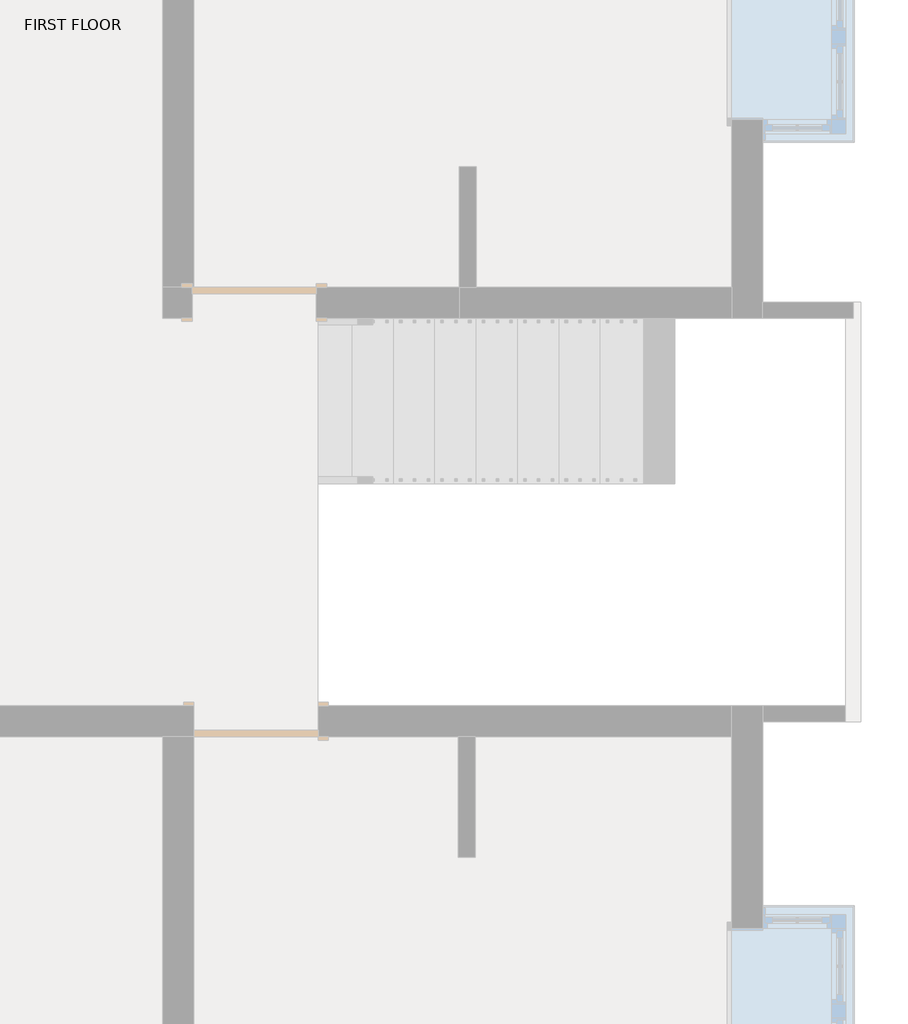
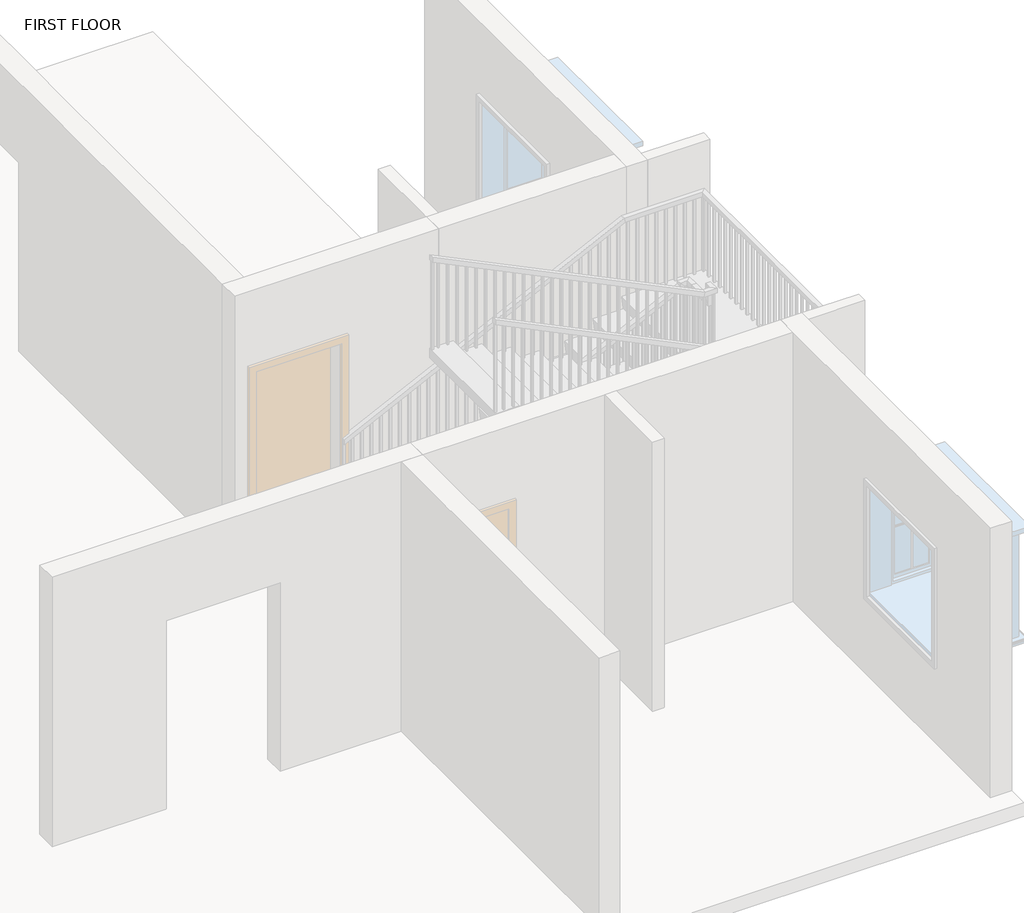
# One storey, part 5 of 6: 1 railing.
"""IFC4 building model written with IfcOpenShell, lengths in millimetres."""

from ifc_helpers import new_model, si_unit, frame, origin, place, context, project, spatial, polyline, outline, extrude, faceted_brep, element, save

model = new_model("IFC4")

# Units and contexts
model_context = context("Model", 3, world=origin())
ifc_project = project(units=[si_unit("LENGTHUNIT", "METRE", prefix="MILLI")], contexts=[model_context])

# Site, building, storey
site = spatial("IfcSite", under=ifc_project)
building = spatial("IfcBuilding", under=site)
storey = spatial("IfcBuildingStorey", under=building, Name="FIRST FLOOR", Elevation=3200.4)

# Railing
placement = place(None, origin())
element("IfcRailing", 1, ObjectType="Handrail - Rectangular", at=placement, inside=storey, context=model_context, shape_type="SolidModel", body=[
    faceted_brep([(3126.2584916, 220.733346, 4260.2727273), (3126.2584916, 220.733346, 4203.7956113), (3126.2584916, 169.933346, 4203.7956113), (3126.2584916, 169.933346, 4260.2727273), (6120.7829507, 220.733346, 5715.0), (6132.4691705, 220.733346, 5664.2), (6132.4691705, 169.933346, 5664.2), (6120.7829507, 169.933346, 5715.0), (7009.1350459, 220.733346, 5715.0), (7009.1350459, 220.733346, 5664.2), (6958.3350459, 169.933346, 5664.2), (6958.3350459, 169.933346, 5715.0), (7009.1350459, -2636.766654, 5715.0), (7009.1350459, -2636.766654, 5664.2), (6958.3350459, -2585.966654, 5664.2), (6958.3350459, -2585.966654, 5715.0), (6420.2353966, -2636.766654, 5715.0), (6408.5491768, -2636.766654, 5664.2), (6408.5491768, -2585.966654, 5664.2), (6420.2353966, -2585.966654, 5715.0), (3126.2584916, -2636.766654, 7315.2), (3126.2584916, -2585.966654, 7315.2), (3126.2584916, -2585.966654, 7258.722884), (3126.2584916, -2636.766654, 7258.722884)], [[[0, 1, 2, 3]], [[1, 0, 4, 5]], [[2, 1, 5, 6]], [[3, 2, 6, 7]], [[0, 3, 7, 4]], [[5, 4, 8, 9]], [[6, 5, 9, 10]], [[7, 6, 10, 11]], [[4, 7, 11, 8]], [[9, 8, 12, 13]], [[10, 9, 13, 14]], [[11, 10, 14, 15]], [[8, 11, 15, 12]], [[13, 12, 16, 17]], [[14, 13, 17, 18]], [[15, 14, 18, 19]], [[12, 15, 19, 16]], [[20, 21, 22, 23]], [[17, 16, 20, 23]], [[18, 17, 23, 22]], [[19, 18, 22, 21]], [[16, 19, 21, 20]]]),
    extrude(outline(polyline([(7215.6077556, 3215.0100459), (6255.3272727, 3215.0100459), (6255.3272727, 3234.0600459), (7206.3533465, 3234.0600459), (7215.6077556, 3215.0100459)])), frame((0.0, -2620.891654, 0.0), z_axis=(0.0, 1.0, 0.0), x_axis=(0.0, 0.0, 1.0)), (0.0, 0.0, 1.0), 19.05),
    extrude(outline(polyline([(7166.2509068, 3316.6100459), (6255.3272727, 3316.6100459), (6255.3272727, 3335.6600459), (7156.9964977, 3335.6600459), (7166.2509068, 3316.6100459)])), frame((0.0, -2620.891654, 0.0), z_axis=(0.0, 1.0, 0.0), x_axis=(0.0, 0.0, 1.0)), (0.0, 0.0, 1.0), 19.05),
    extrude(outline(polyline([(7116.894058, 3418.2100459), (6109.8545455, 3418.2100459), (6109.8545455, 3437.2600459), (7107.6396489, 3437.2600459), (7116.894058, 3418.2100459)])), frame((0.0, -2620.891654, 0.0), z_axis=(0.0, 1.0, 0.0), x_axis=(0.0, 0.0, 1.0)), (0.0, 0.0, 1.0), 19.05),
    extrude(outline(polyline([(7067.5372093, 3519.8100459), (6109.8545455, 3519.8100459), (6109.8545455, 3538.8600459), (7058.2828001, 3538.8600459), (7067.5372093, 3519.8100459)])), frame((0.0, -2620.891654, 0.0), z_axis=(0.0, 1.0, 0.0), x_axis=(0.0, 0.0, 1.0)), (0.0, 0.0, 1.0), 19.05),
    extrude(outline(polyline([(7018.1803605, 3621.4100459), (6109.8545455, 3621.4100459), (6109.8545455, 3640.4600459), (7008.9259513, 3640.4600459), (7018.1803605, 3621.4100459)])), frame((0.0, -2620.891654, 0.0), z_axis=(0.0, 1.0, 0.0), x_axis=(0.0, 0.0, 1.0)), (0.0, 0.0, 1.0), 19.05),
    extrude(outline(polyline([(6968.8235117, 3723.0100459), (5964.3818182, 3723.0100459), (5964.3818182, 3742.0600459), (6959.5691025, 3742.0600459), (6968.8235117, 3723.0100459)])), frame((0.0, -2620.891654, 0.0), z_axis=(0.0, 1.0, 0.0), x_axis=(0.0, 0.0, 1.0)), (0.0, 0.0, 1.0), 19.05),
    extrude(outline(polyline([(6919.4666629, 3824.6100459), (5964.3818182, 3824.6100459), (5964.3818182, 3843.6600459), (6910.2122538, 3843.6600459), (6919.4666629, 3824.6100459)])), frame((0.0, -2620.891654, 0.0), z_axis=(0.0, 1.0, 0.0), x_axis=(0.0, 0.0, 1.0)), (0.0, 0.0, 1.0), 19.05),
    extrude(outline(polyline([(6870.1098141, 3926.2100459), (5964.3818182, 3926.2100459), (5964.3818182, 3945.2600459), (6860.855405, 3945.2600459), (6870.1098141, 3926.2100459)])), frame((0.0, -2620.891654, 0.0), z_axis=(0.0, 1.0, 0.0), x_axis=(0.0, 0.0, 1.0)), (0.0, 0.0, 1.0), 19.05),
    extrude(outline(polyline([(6820.7529653, 4027.8100459), (5818.9090909, 4027.8100459), (5818.9090909, 4046.8600459), (6811.4985562, 4046.8600459), (6820.7529653, 4027.8100459)])), frame((0.0, -2620.891654, 0.0), z_axis=(0.0, 1.0, 0.0), x_axis=(0.0, 0.0, 1.0)), (0.0, 0.0, 1.0), 19.05),
    extrude(outline(polyline([(6771.3961165, 4129.4100459), (5818.9090909, 4129.4100459), (5818.9090909, 4148.4600459), (6762.1417074, 4148.4600459), (6771.3961165, 4129.4100459)])), frame((0.0, -2620.891654, 0.0), z_axis=(0.0, 1.0, 0.0), x_axis=(0.0, 0.0, 1.0)), (0.0, 0.0, 1.0), 19.05),
    extrude(outline(polyline([(6722.0392678, 4231.0100459), (5818.9090909, 4231.0100459), (5818.9090909, 4250.0600459), (6712.7848586, 4250.0600459), (6722.0392678, 4231.0100459)])), frame((0.0, -2620.891654, 0.0), z_axis=(0.0, 1.0, 0.0), x_axis=(0.0, 0.0, 1.0)), (0.0, 0.0, 1.0), 19.05),
    extrude(outline(polyline([(6672.682419, 4332.6100459), (5673.4363636, 4332.6100459), (5673.4363636, 4351.6600459), (6663.4280098, 4351.6600459), (6672.682419, 4332.6100459)])), frame((0.0, -2620.891654, 0.0), z_axis=(0.0, 1.0, 0.0), x_axis=(0.0, 0.0, 1.0)), (0.0, 0.0, 1.0), 19.05),
    extrude(outline(polyline([(6623.3255702, 4434.2100459), (5673.4363636, 4434.2100459), (5673.4363636, 4453.2600459), (6614.071161, 4453.2600459), (6623.3255702, 4434.2100459)])), frame((0.0, -2620.891654, 0.0), z_axis=(0.0, 1.0, 0.0), x_axis=(0.0, 0.0, 1.0)), (0.0, 0.0, 1.0), 19.05),
    extrude(outline(polyline([(6573.9687214, 4535.8100459), (5673.4363636, 4535.8100459), (5673.4363636, 4554.8600459), (6564.7143123, 4554.8600459), (6573.9687214, 4535.8100459)])), frame((0.0, -2620.891654, 0.0), z_axis=(0.0, 1.0, 0.0), x_axis=(0.0, 0.0, 1.0)), (0.0, 0.0, 1.0), 19.05),
    extrude(outline(polyline([(6524.6118726, 4637.4100459), (5527.9636364, 4637.4100459), (5527.9636364, 4656.4600459), (6515.3574635, 4656.4600459), (6524.6118726, 4637.4100459)])), frame((0.0, -2620.891654, 0.0), z_axis=(0.0, 1.0, 0.0), x_axis=(0.0, 0.0, 1.0)), (0.0, 0.0, 1.0), 19.05),
    extrude(outline(polyline([(6475.2550238, 4739.0100459), (5527.9636364, 4739.0100459), (5527.9636364, 4758.0600459), (6466.0006147, 4758.0600459), (6475.2550238, 4739.0100459)])), frame((0.0, -2620.891654, 0.0), z_axis=(0.0, 1.0, 0.0), x_axis=(0.0, 0.0, 1.0)), (0.0, 0.0, 1.0), 19.05),
    extrude(outline(polyline([(6425.8981751, 4840.6100459), (5527.9636364, 4840.6100459), (5527.9636364, 4859.6600459), (6416.6437659, 4859.6600459), (6425.8981751, 4840.6100459)])), frame((0.0, -2620.891654, 0.0), z_axis=(0.0, 1.0, 0.0), x_axis=(0.0, 0.0, 1.0)), (0.0, 0.0, 1.0), 19.05),
    extrude(outline(polyline([(6376.5413263, 4942.2100459), (5382.4909091, 4942.2100459), (5382.4909091, 4961.2600459), (6367.2869171, 4961.2600459), (6376.5413263, 4942.2100459)])), frame((0.0, -2620.891654, 0.0), z_axis=(0.0, 1.0, 0.0), x_axis=(0.0, 0.0, 1.0)), (0.0, 0.0, 1.0), 19.05),
    extrude(outline(polyline([(6327.1844775, 5043.8100459), (5382.4909091, 5043.8100459), (5382.4909091, 5062.8600459), (6317.9300683, 5062.8600459), (6327.1844775, 5043.8100459)])), frame((0.0, -2620.891654, 0.0), z_axis=(0.0, 1.0, 0.0), x_axis=(0.0, 0.0, 1.0)), (0.0, 0.0, 1.0), 19.05),
    extrude(outline(polyline([(6277.8276287, 5145.4100459), (5382.4909091, 5145.4100459), (5382.4909091, 5164.4600459), (6268.5732196, 5164.4600459), (6277.8276287, 5145.4100459)])), frame((0.0, -2620.891654, 0.0), z_axis=(0.0, 1.0, 0.0), x_axis=(0.0, 0.0, 1.0)), (0.0, 0.0, 1.0), 19.05),
    extrude(outline(polyline([(6228.4707799, 5247.0100459), (5237.0181818, 5247.0100459), (5237.0181818, 5266.0600459), (6219.2163708, 5266.0600459), (6228.4707799, 5247.0100459)])), frame((0.0, -2620.891654, 0.0), z_axis=(0.0, 1.0, 0.0), x_axis=(0.0, 0.0, 1.0)), (0.0, 0.0, 1.0), 19.05),
    extrude(outline(polyline([(6179.1139311, 5348.6100459), (5237.0181818, 5348.6100459), (5237.0181818, 5367.6600459), (6169.859522, 5367.6600459), (6179.1139311, 5348.6100459)])), frame((0.0, -2620.891654, 0.0), z_axis=(0.0, 1.0, 0.0), x_axis=(0.0, 0.0, 1.0)), (0.0, 0.0, 1.0), 19.05),
    extrude(outline(polyline([(6129.7570823, 5450.2100459), (5237.0181818, 5450.2100459), (5237.0181818, 5469.2600459), (6120.5026732, 5469.2600459), (6129.7570823, 5450.2100459)])), frame((0.0, -2620.891654, 0.0), z_axis=(0.0, 1.0, 0.0), x_axis=(0.0, 0.0, 1.0)), (0.0, 0.0, 1.0), 19.05),
    extrude(outline(polyline([(6080.4002336, 5551.8100459), (5091.5454545, 5551.8100459), (5091.5454545, 5570.8600459), (6071.1458244, 5570.8600459), (6080.4002336, 5551.8100459)])), frame((0.0, -2620.891654, 0.0), z_axis=(0.0, 1.0, 0.0), x_axis=(0.0, 0.0, 1.0)), (0.0, 0.0, 1.0), 19.05),
    extrude(outline(polyline([(6031.0433848, 5653.4100459), (5091.5454545, 5653.4100459), (5091.5454545, 5672.4600459), (6021.7889756, 5672.4600459), (6031.0433848, 5653.4100459)])), frame((0.0, -2620.891654, 0.0), z_axis=(0.0, 1.0, 0.0), x_axis=(0.0, 0.0, 1.0)), (0.0, 0.0, 1.0), 19.05),
    extrude(outline(polyline([(5981.686536, 5755.0100459), (5091.5454545, 5755.0100459), (5091.5454545, 5774.0600459), (5972.4321268, 5774.0600459), (5981.686536, 5755.0100459)])), frame((0.0, -2620.891654, 0.0), z_axis=(0.0, 1.0, 0.0), x_axis=(0.0, 0.0, 1.0)), (0.0, 0.0, 1.0), 19.05),
    extrude(outline(polyline([(5932.3296872, 5856.6100459), (4946.0727273, 5856.6100459), (4946.0727273, 5875.6600459), (5923.0752781, 5875.6600459), (5932.3296872, 5856.6100459)])), frame((0.0, -2620.891654, 0.0), z_axis=(0.0, 1.0, 0.0), x_axis=(0.0, 0.0, 1.0)), (0.0, 0.0, 1.0), 19.05),
    extrude(outline(polyline([(5882.9728384, 5958.2100459), (4946.0727273, 5958.2100459), (4946.0727273, 5977.2600459), (5873.7184293, 5977.2600459), (5882.9728384, 5958.2100459)])), frame((0.0, -2620.891654, 0.0), z_axis=(0.0, 1.0, 0.0), x_axis=(0.0, 0.0, 1.0)), (0.0, 0.0, 1.0), 19.05),
    extrude(outline(polyline([(5833.6159896, 6059.8100459), (4946.0727273, 6059.8100459), (4946.0727273, 6078.8600459), (5824.3615805, 6078.8600459), (5833.6159896, 6059.8100459)])), frame((0.0, -2620.891654, 0.0), z_axis=(0.0, 1.0, 0.0), x_axis=(0.0, 0.0, 1.0)), (0.0, 0.0, 1.0), 19.05),
    extrude(outline(polyline([(5784.2591409, 6161.4100459), (4800.6, 6161.4100459), (4800.6, 6180.4600459), (5775.0047317, 6180.4600459), (5784.2591409, 6161.4100459)])), frame((0.0, -2620.891654, 0.0), z_axis=(0.0, 1.0, 0.0), x_axis=(0.0, 0.0, 1.0)), (0.0, 0.0, 1.0), 19.05),
    extrude(outline(polyline([(5734.9022921, 6263.0100459), (4800.6, 6263.0100459), (4800.6, 6282.0600459), (5725.6478829, 6282.0600459), (5734.9022921, 6263.0100459)])), frame((0.0, -2620.891654, 0.0), z_axis=(0.0, 1.0, 0.0), x_axis=(0.0, 0.0, 1.0)), (0.0, 0.0, 1.0), 19.05),
    extrude(outline(polyline([(5685.5454433, 6364.6100459), (4800.6, 6364.6100459), (4800.6, 6383.6600459), (5676.2910341, 6383.6600459), (5685.5454433, 6364.6100459)])), frame((0.0, -2620.891654, 0.0), z_axis=(0.0, 1.0, 0.0), x_axis=(0.0, 0.0, 1.0)), (0.0, 0.0, 1.0), 19.05),
    extrude(outline(polyline([(6485.2600459, -2620.891654), (6466.2100459, -2620.891654), (6466.2100459, -2601.841654), (6485.2600459, -2601.841654), (6485.2600459, -2620.891654)])), frame((0.0, 0.0, 4800.6), z_axis=(0.0, 0.0, 1.0), x_axis=(1.0, 0.0, 0.0)), (0.0, 0.0, 1.0), 863.6),
    extrude(outline(polyline([(6586.8600459, -2620.891654), (6567.8100459, -2620.891654), (6567.8100459, -2601.841654), (6586.8600459, -2601.841654), (6586.8600459, -2620.891654)])), frame((0.0, 0.0, 4800.6), z_axis=(0.0, 0.0, 1.0), x_axis=(1.0, 0.0, 0.0)), (0.0, 0.0, 1.0), 863.6),
    extrude(outline(polyline([(6688.4600459, -2620.891654), (6669.4100459, -2620.891654), (6669.4100459, -2601.841654), (6688.4600459, -2601.841654), (6688.4600459, -2620.891654)])), frame((0.0, 0.0, 4800.6), z_axis=(0.0, 0.0, 1.0), x_axis=(1.0, 0.0, 0.0)), (0.0, 0.0, 1.0), 863.6),
    extrude(outline(polyline([(6790.0600459, -2620.891654), (6771.0100459, -2620.891654), (6771.0100459, -2601.841654), (6790.0600459, -2601.841654), (6790.0600459, -2620.891654)])), frame((0.0, 0.0, 4800.6), z_axis=(0.0, 0.0, 1.0), x_axis=(1.0, 0.0, 0.0)), (0.0, 0.0, 1.0), 863.6),
    extrude(outline(polyline([(6891.6600459, -2620.891654), (6872.6100459, -2620.891654), (6872.6100459, -2601.841654), (6891.6600459, -2601.841654), (6891.6600459, -2620.891654)])), frame((0.0, 0.0, 4800.6), z_axis=(0.0, 0.0, 1.0), x_axis=(1.0, 0.0, 0.0)), (0.0, 0.0, 1.0), 863.6),
    extrude(outline(polyline([(6993.2600459, -2538.341654), (6993.2600459, -2557.391654), (6974.2100459, -2557.391654), (6974.2100459, -2538.341654), (6993.2600459, -2538.341654)])), frame((0.0, 0.0, 4800.6), z_axis=(0.0, 0.0, 1.0), x_axis=(1.0, 0.0, 0.0)), (0.0, 0.0, 1.0), 863.6),
    extrude(outline(polyline([(6993.2600459, -2436.741654), (6993.2600459, -2455.791654), (6974.2100459, -2455.791654), (6974.2100459, -2436.741654), (6993.2600459, -2436.741654)])), frame((0.0, 0.0, 4800.6), z_axis=(0.0, 0.0, 1.0), x_axis=(1.0, 0.0, 0.0)), (0.0, 0.0, 1.0), 863.6),
    extrude(outline(polyline([(6993.2600459, -2335.141654), (6993.2600459, -2354.191654), (6974.2100459, -2354.191654), (6974.2100459, -2335.141654), (6993.2600459, -2335.141654)])), frame((0.0, 0.0, 4800.6), z_axis=(0.0, 0.0, 1.0), x_axis=(1.0, 0.0, 0.0)), (0.0, 0.0, 1.0), 863.6),
    extrude(outline(polyline([(6993.2600459, -2233.541654), (6993.2600459, -2252.591654), (6974.2100459, -2252.591654), (6974.2100459, -2233.541654), (6993.2600459, -2233.541654)])), frame((0.0, 0.0, 4800.6), z_axis=(0.0, 0.0, 1.0), x_axis=(1.0, 0.0, 0.0)), (0.0, 0.0, 1.0), 863.6),
    extrude(outline(polyline([(6993.2600459, -2131.941654), (6993.2600459, -2150.991654), (6974.2100459, -2150.991654), (6974.2100459, -2131.941654), (6993.2600459, -2131.941654)])), frame((0.0, 0.0, 4800.6), z_axis=(0.0, 0.0, 1.0), x_axis=(1.0, 0.0, 0.0)), (0.0, 0.0, 1.0), 863.6),
    extrude(outline(polyline([(6993.2600459, -2030.341654), (6993.2600459, -2049.391654), (6974.2100459, -2049.391654), (6974.2100459, -2030.341654), (6993.2600459, -2030.341654)])), frame((0.0, 0.0, 4800.6), z_axis=(0.0, 0.0, 1.0), x_axis=(1.0, 0.0, 0.0)), (0.0, 0.0, 1.0), 863.6),
    extrude(outline(polyline([(6993.2600459, -1928.741654), (6993.2600459, -1947.791654), (6974.2100459, -1947.791654), (6974.2100459, -1928.741654), (6993.2600459, -1928.741654)])), frame((0.0, 0.0, 4800.6), z_axis=(0.0, 0.0, 1.0), x_axis=(1.0, 0.0, 0.0)), (0.0, 0.0, 1.0), 863.6),
    extrude(outline(polyline([(6993.2600459, -1827.141654), (6993.2600459, -1846.191654), (6974.2100459, -1846.191654), (6974.2100459, -1827.141654), (6993.2600459, -1827.141654)])), frame((0.0, 0.0, 4800.6), z_axis=(0.0, 0.0, 1.0), x_axis=(1.0, 0.0, 0.0)), (0.0, 0.0, 1.0), 863.6),
    extrude(outline(polyline([(6993.2600459, -1725.541654), (6993.2600459, -1744.591654), (6974.2100459, -1744.591654), (6974.2100459, -1725.541654), (6993.2600459, -1725.541654)])), frame((0.0, 0.0, 4800.6), z_axis=(0.0, 0.0, 1.0), x_axis=(1.0, 0.0, 0.0)), (0.0, 0.0, 1.0), 863.6),
    extrude(outline(polyline([(6993.2600459, -1623.941654), (6993.2600459, -1642.991654), (6974.2100459, -1642.991654), (6974.2100459, -1623.941654), (6993.2600459, -1623.941654)])), frame((0.0, 0.0, 4800.6), z_axis=(0.0, 0.0, 1.0), x_axis=(1.0, 0.0, 0.0)), (0.0, 0.0, 1.0), 863.6),
    extrude(outline(polyline([(6993.2600459, -1522.341654), (6993.2600459, -1541.391654), (6974.2100459, -1541.391654), (6974.2100459, -1522.341654), (6993.2600459, -1522.341654)])), frame((0.0, 0.0, 4800.6), z_axis=(0.0, 0.0, 1.0), x_axis=(1.0, 0.0, 0.0)), (0.0, 0.0, 1.0), 863.6),
    extrude(outline(polyline([(6993.2600459, -1420.741654), (6993.2600459, -1439.791654), (6974.2100459, -1439.791654), (6974.2100459, -1420.741654), (6993.2600459, -1420.741654)])), frame((0.0, 0.0, 4800.6), z_axis=(0.0, 0.0, 1.0), x_axis=(1.0, 0.0, 0.0)), (0.0, 0.0, 1.0), 863.6),
    extrude(outline(polyline([(6993.2600459, -1319.141654), (6993.2600459, -1338.191654), (6974.2100459, -1338.191654), (6974.2100459, -1319.141654), (6993.2600459, -1319.141654)])), frame((0.0, 0.0, 4800.6), z_axis=(0.0, 0.0, 1.0), x_axis=(1.0, 0.0, 0.0)), (0.0, 0.0, 1.0), 863.6),
    extrude(outline(polyline([(6993.2600459, -1217.541654), (6993.2600459, -1236.591654), (6974.2100459, -1236.591654), (6974.2100459, -1217.541654), (6993.2600459, -1217.541654)])), frame((0.0, 0.0, 4800.6), z_axis=(0.0, 0.0, 1.0), x_axis=(1.0, 0.0, 0.0)), (0.0, 0.0, 1.0), 863.6),
    extrude(outline(polyline([(6993.2600459, -1115.941654), (6993.2600459, -1134.991654), (6974.2100459, -1134.991654), (6974.2100459, -1115.941654), (6993.2600459, -1115.941654)])), frame((0.0, 0.0, 4800.6), z_axis=(0.0, 0.0, 1.0), x_axis=(1.0, 0.0, 0.0)), (0.0, 0.0, 1.0), 863.6),
    extrude(outline(polyline([(6993.2600459, -1014.341654), (6993.2600459, -1033.391654), (6974.2100459, -1033.391654), (6974.2100459, -1014.341654), (6993.2600459, -1014.341654)])), frame((0.0, 0.0, 4800.6), z_axis=(0.0, 0.0, 1.0), x_axis=(1.0, 0.0, 0.0)), (0.0, 0.0, 1.0), 863.6),
    extrude(outline(polyline([(6993.2600459, -912.741654), (6993.2600459, -931.791654), (6974.2100459, -931.791654), (6974.2100459, -912.741654), (6993.2600459, -912.741654)])), frame((0.0, 0.0, 4800.6), z_axis=(0.0, 0.0, 1.0), x_axis=(1.0, 0.0, 0.0)), (0.0, 0.0, 1.0), 863.6),
    extrude(outline(polyline([(6993.2600459, -811.141654), (6993.2600459, -830.191654), (6974.2100459, -830.191654), (6974.2100459, -811.141654), (6993.2600459, -811.141654)])), frame((0.0, 0.0, 4800.6), z_axis=(0.0, 0.0, 1.0), x_axis=(1.0, 0.0, 0.0)), (0.0, 0.0, 1.0), 863.6),
    extrude(outline(polyline([(6993.2600459, -709.541654), (6993.2600459, -728.591654), (6974.2100459, -728.591654), (6974.2100459, -709.541654), (6993.2600459, -709.541654)])), frame((0.0, 0.0, 4800.6), z_axis=(0.0, 0.0, 1.0), x_axis=(1.0, 0.0, 0.0)), (0.0, 0.0, 1.0), 863.6),
    extrude(outline(polyline([(6993.2600459, -607.941654), (6993.2600459, -626.991654), (6974.2100459, -626.991654), (6974.2100459, -607.941654), (6993.2600459, -607.941654)])), frame((0.0, 0.0, 4800.6), z_axis=(0.0, 0.0, 1.0), x_axis=(1.0, 0.0, 0.0)), (0.0, 0.0, 1.0), 863.6),
    extrude(outline(polyline([(6993.2600459, -506.341654), (6993.2600459, -525.391654), (6974.2100459, -525.391654), (6974.2100459, -506.341654), (6993.2600459, -506.341654)])), frame((0.0, 0.0, 4800.6), z_axis=(0.0, 0.0, 1.0), x_axis=(1.0, 0.0, 0.0)), (0.0, 0.0, 1.0), 863.6),
    extrude(outline(polyline([(6993.2600459, -404.741654), (6993.2600459, -423.791654), (6974.2100459, -423.791654), (6974.2100459, -404.741654), (6993.2600459, -404.741654)])), frame((0.0, 0.0, 4800.6), z_axis=(0.0, 0.0, 1.0), x_axis=(1.0, 0.0, 0.0)), (0.0, 0.0, 1.0), 863.6),
    extrude(outline(polyline([(6993.2600459, -303.141654), (6993.2600459, -322.191654), (6974.2100459, -322.191654), (6974.2100459, -303.141654), (6993.2600459, -303.141654)])), frame((0.0, 0.0, 4800.6), z_axis=(0.0, 0.0, 1.0), x_axis=(1.0, 0.0, 0.0)), (0.0, 0.0, 1.0), 863.6),
    extrude(outline(polyline([(6993.2600459, -201.541654), (6993.2600459, -220.591654), (6974.2100459, -220.591654), (6974.2100459, -201.541654), (6993.2600459, -201.541654)])), frame((0.0, 0.0, 4800.6), z_axis=(0.0, 0.0, 1.0), x_axis=(1.0, 0.0, 0.0)), (0.0, 0.0, 1.0), 863.6),
    extrude(outline(polyline([(6993.2600459, -99.941654), (6993.2600459, -118.991654), (6974.2100459, -118.991654), (6974.2100459, -99.941654), (6993.2600459, -99.941654)])), frame((0.0, 0.0, 4800.6), z_axis=(0.0, 0.0, 1.0), x_axis=(1.0, 0.0, 0.0)), (0.0, 0.0, 1.0), 863.6),
    extrude(outline(polyline([(6993.2600459, 1.658346), (6993.2600459, -17.391654), (6974.2100459, -17.391654), (6974.2100459, 1.658346), (6993.2600459, 1.658346)])), frame((0.0, 0.0, 4800.6), z_axis=(0.0, 0.0, 1.0), x_axis=(1.0, 0.0, 0.0)), (0.0, 0.0, 1.0), 863.6),
    extrude(outline(polyline([(6993.2600459, 103.258346), (6993.2600459, 84.208346), (6974.2100459, 84.208346), (6974.2100459, 103.258346), (6993.2600459, 103.258346)])), frame((0.0, 0.0, 4800.6), z_axis=(0.0, 0.0, 1.0), x_axis=(1.0, 0.0, 0.0)), (0.0, 0.0, 1.0), 863.6),
    extrude(outline(polyline([(6875.9334916, 204.858346), (6894.9834916, 204.858346), (6894.9834916, 185.808346), (6875.9334916, 185.808346), (6875.9334916, 204.858346)])), frame((0.0, 0.0, 4800.6), z_axis=(0.0, 0.0, 1.0), x_axis=(1.0, 0.0, 0.0)), (0.0, 0.0, 1.0), 863.6),
    extrude(outline(polyline([(6774.3334916, 204.858346), (6793.3834916, 204.858346), (6793.3834916, 185.808346), (6774.3334916, 185.808346), (6774.3334916, 204.858346)])), frame((0.0, 0.0, 4800.6), z_axis=(0.0, 0.0, 1.0), x_axis=(1.0, 0.0, 0.0)), (0.0, 0.0, 1.0), 863.6),
    extrude(outline(polyline([(6672.7334916, 204.858346), (6691.7834916, 204.858346), (6691.7834916, 185.808346), (6672.7334916, 185.808346), (6672.7334916, 204.858346)])), frame((0.0, 0.0, 4800.6), z_axis=(0.0, 0.0, 1.0), x_axis=(1.0, 0.0, 0.0)), (0.0, 0.0, 1.0), 863.6),
    extrude(outline(polyline([(6571.1334916, 204.858346), (6590.1834916, 204.858346), (6590.1834916, 185.808346), (6571.1334916, 185.808346), (6571.1334916, 204.858346)])), frame((0.0, 0.0, 4800.6), z_axis=(0.0, 0.0, 1.0), x_axis=(1.0, 0.0, 0.0)), (0.0, 0.0, 1.0), 863.6),
    extrude(outline(polyline([(6469.5334916, 204.858346), (6488.5834916, 204.858346), (6488.5834916, 185.808346), (6469.5334916, 185.808346), (6469.5334916, 204.858346)])), frame((0.0, 0.0, 4800.6), z_axis=(0.0, 0.0, 1.0), x_axis=(1.0, 0.0, 0.0)), (0.0, 0.0, 1.0), 863.6),
    extrude(outline(polyline([(6367.9334916, 204.858346), (6386.9834916, 204.858346), (6386.9834916, 185.808346), (6367.9334916, 185.808346), (6367.9334916, 204.858346)])), frame((0.0, 0.0, 4800.6), z_axis=(0.0, 0.0, 1.0), x_axis=(1.0, 0.0, 0.0)), (0.0, 0.0, 1.0), 863.6),
    extrude(outline(polyline([(6266.3334916, 204.858346), (6285.3834916, 204.858346), (6285.3834916, 185.808346), (6266.3334916, 185.808346), (6266.3334916, 204.858346)])), frame((0.0, 0.0, 4800.6), z_axis=(0.0, 0.0, 1.0), x_axis=(1.0, 0.0, 0.0)), (0.0, 0.0, 1.0), 863.6),
    extrude(outline(polyline([(6164.7334916, 204.858346), (6183.7834916, 204.858346), (6183.7834916, 185.808346), (6164.7334916, 185.808346), (6164.7334916, 204.858346)])), frame((0.0, 0.0, 4800.6), z_axis=(0.0, 0.0, 1.0), x_axis=(1.0, 0.0, 0.0)), (0.0, 0.0, 1.0), 863.6),
    extrude(outline(polyline([(5630.5170215, 6063.1334916), (4655.1272727, 6063.1334916), (4655.1272727, 6082.1834916), (5639.7714306, 6082.1834916), (5630.5170215, 6063.1334916)])), frame((0.0, 185.808346, 0.0), z_axis=(0.0, 1.0, 0.0), x_axis=(0.0, 0.0, 1.0)), (0.0, 0.0, 1.0), 19.05),
    extrude(outline(polyline([(5581.1601727, 5961.5334916), (4655.1272727, 5961.5334916), (4655.1272727, 5980.5834916), (5590.4145818, 5980.5834916), (5581.1601727, 5961.5334916)])), frame((0.0, 185.808346, 0.0), z_axis=(0.0, 1.0, 0.0), x_axis=(0.0, 0.0, 1.0)), (0.0, 0.0, 1.0), 19.05),
    extrude(outline(polyline([(5531.8033239, 5859.9334916), (4655.1272727, 5859.9334916), (4655.1272727, 5878.9834916), (5541.057733, 5878.9834916), (5531.8033239, 5859.9334916)])), frame((0.0, 185.808346, 0.0), z_axis=(0.0, 1.0, 0.0), x_axis=(0.0, 0.0, 1.0)), (0.0, 0.0, 1.0), 19.05),
    extrude(outline(polyline([(5482.4464751, 5758.3334916), (4509.6545455, 5758.3334916), (4509.6545455, 5777.3834916), (5491.7008843, 5777.3834916), (5482.4464751, 5758.3334916)])), frame((0.0, 185.808346, 0.0), z_axis=(0.0, 1.0, 0.0), x_axis=(0.0, 0.0, 1.0)), (0.0, 0.0, 1.0), 19.05),
    extrude(outline(polyline([(5433.0896263, 5656.7334916), (4509.6545455, 5656.7334916), (4509.6545455, 5675.7834916), (5442.3440355, 5675.7834916), (5433.0896263, 5656.7334916)])), frame((0.0, 185.808346, 0.0), z_axis=(0.0, 1.0, 0.0), x_axis=(0.0, 0.0, 1.0)), (0.0, 0.0, 1.0), 19.05),
    extrude(outline(polyline([(5383.7327775, 5555.1334916), (4509.6545455, 5555.1334916), (4509.6545455, 5574.1834916), (5392.9871867, 5574.1834916), (5383.7327775, 5555.1334916)])), frame((0.0, 185.808346, 0.0), z_axis=(0.0, 1.0, 0.0), x_axis=(0.0, 0.0, 1.0)), (0.0, 0.0, 1.0), 19.05),
    extrude(outline(polyline([(5334.3759288, 5453.5334916), (4364.1818182, 5453.5334916), (4364.1818182, 5472.5834916), (5343.6303379, 5472.5834916), (5334.3759288, 5453.5334916)])), frame((0.0, 185.808346, 0.0), z_axis=(0.0, 1.0, 0.0), x_axis=(0.0, 0.0, 1.0)), (0.0, 0.0, 1.0), 19.05),
    extrude(outline(polyline([(5285.01908, 5351.9334916), (4364.1818182, 5351.9334916), (4364.1818182, 5370.9834916), (5294.2734891, 5370.9834916), (5285.01908, 5351.9334916)])), frame((0.0, 185.808346, 0.0), z_axis=(0.0, 1.0, 0.0), x_axis=(0.0, 0.0, 1.0)), (0.0, 0.0, 1.0), 19.05),
    extrude(outline(polyline([(5235.6622312, 5250.3334916), (4364.1818182, 5250.3334916), (4364.1818182, 5269.3834916), (5244.9166403, 5269.3834916), (5235.6622312, 5250.3334916)])), frame((0.0, 185.808346, 0.0), z_axis=(0.0, 1.0, 0.0), x_axis=(0.0, 0.0, 1.0)), (0.0, 0.0, 1.0), 19.05),
    extrude(outline(polyline([(5186.3053824, 5148.7334916), (4218.7090909, 5148.7334916), (4218.7090909, 5167.7834916), (5195.5597915, 5167.7834916), (5186.3053824, 5148.7334916)])), frame((0.0, 185.808346, 0.0), z_axis=(0.0, 1.0, 0.0), x_axis=(0.0, 0.0, 1.0)), (0.0, 0.0, 1.0), 19.05),
    extrude(outline(polyline([(5136.9485336, 5047.1334916), (4218.7090909, 5047.1334916), (4218.7090909, 5066.1834916), (5146.2029428, 5066.1834916), (5136.9485336, 5047.1334916)])), frame((0.0, 185.808346, 0.0), z_axis=(0.0, 1.0, 0.0), x_axis=(0.0, 0.0, 1.0)), (0.0, 0.0, 1.0), 19.05),
    extrude(outline(polyline([(5087.5916848, 4945.5334916), (4218.7090909, 4945.5334916), (4218.7090909, 4964.5834916), (5096.846094, 4964.5834916), (5087.5916848, 4945.5334916)])), frame((0.0, 185.808346, 0.0), z_axis=(0.0, 1.0, 0.0), x_axis=(0.0, 0.0, 1.0)), (0.0, 0.0, 1.0), 19.05),
    extrude(outline(polyline([(5038.234836, 4843.9334916), (4073.2363636, 4843.9334916), (4073.2363636, 4862.9834916), (5047.4892452, 4862.9834916), (5038.234836, 4843.9334916)])), frame((0.0, 185.808346, 0.0), z_axis=(0.0, 1.0, 0.0), x_axis=(0.0, 0.0, 1.0)), (0.0, 0.0, 1.0), 19.05),
    extrude(outline(polyline([(4988.8779873, 4742.3334916), (4073.2363636, 4742.3334916), (4073.2363636, 4761.3834916), (4998.1323964, 4761.3834916), (4988.8779873, 4742.3334916)])), frame((0.0, 185.808346, 0.0), z_axis=(0.0, 1.0, 0.0), x_axis=(0.0, 0.0, 1.0)), (0.0, 0.0, 1.0), 19.05),
    extrude(outline(polyline([(4939.5211385, 4640.7334916), (4073.2363636, 4640.7334916), (4073.2363636, 4659.7834916), (4948.7755476, 4659.7834916), (4939.5211385, 4640.7334916)])), frame((0.0, 185.808346, 0.0), z_axis=(0.0, 1.0, 0.0), x_axis=(0.0, 0.0, 1.0)), (0.0, 0.0, 1.0), 19.05),
    extrude(outline(polyline([(4890.1642897, 4539.1334916), (3927.7636364, 4539.1334916), (3927.7636364, 4558.1834916), (4899.4186988, 4558.1834916), (4890.1642897, 4539.1334916)])), frame((0.0, 185.808346, 0.0), z_axis=(0.0, 1.0, 0.0), x_axis=(0.0, 0.0, 1.0)), (0.0, 0.0, 1.0), 19.05),
    extrude(outline(polyline([(4840.8074409, 4437.5334916), (3927.7636364, 4437.5334916), (3927.7636364, 4456.5834916), (4850.0618501, 4456.5834916), (4840.8074409, 4437.5334916)])), frame((0.0, 185.808346, 0.0), z_axis=(0.0, 1.0, 0.0), x_axis=(0.0, 0.0, 1.0)), (0.0, 0.0, 1.0), 19.05),
    extrude(outline(polyline([(4791.4505921, 4335.9334916), (3927.7636364, 4335.9334916), (3927.7636364, 4354.9834916), (4800.7050013, 4354.9834916), (4791.4505921, 4335.9334916)])), frame((0.0, 185.808346, 0.0), z_axis=(0.0, 1.0, 0.0), x_axis=(0.0, 0.0, 1.0)), (0.0, 0.0, 1.0), 19.05),
    extrude(outline(polyline([(4742.0937433, 4234.3334916), (3782.2909091, 4234.3334916), (3782.2909091, 4253.3834916), (4751.3481525, 4253.3834916), (4742.0937433, 4234.3334916)])), frame((0.0, 185.808346, 0.0), z_axis=(0.0, 1.0, 0.0), x_axis=(0.0, 0.0, 1.0)), (0.0, 0.0, 1.0), 19.05),
    extrude(outline(polyline([(4692.7368946, 4132.7334916), (3782.2909091, 4132.7334916), (3782.2909091, 4151.7834916), (4701.9913037, 4151.7834916), (4692.7368946, 4132.7334916)])), frame((0.0, 185.808346, 0.0), z_axis=(0.0, 1.0, 0.0), x_axis=(0.0, 0.0, 1.0)), (0.0, 0.0, 1.0), 19.05),
    extrude(outline(polyline([(4643.3800458, 4031.1334916), (3782.2909091, 4031.1334916), (3782.2909091, 4050.1834916), (4652.6344549, 4050.1834916), (4643.3800458, 4031.1334916)])), frame((0.0, 185.808346, 0.0), z_axis=(0.0, 1.0, 0.0), x_axis=(0.0, 0.0, 1.0)), (0.0, 0.0, 1.0), 19.05),
    extrude(outline(polyline([(4594.023197, 3929.5334916), (3636.8181818, 3929.5334916), (3636.8181818, 3948.5834916), (4603.2776061, 3948.5834916), (4594.023197, 3929.5334916)])), frame((0.0, 185.808346, 0.0), z_axis=(0.0, 1.0, 0.0), x_axis=(0.0, 0.0, 1.0)), (0.0, 0.0, 1.0), 19.05),
    extrude(outline(polyline([(4544.6663482, 3827.9334916), (3636.8181818, 3827.9334916), (3636.8181818, 3846.9834916), (4553.9207573, 3846.9834916), (4544.6663482, 3827.9334916)])), frame((0.0, 185.808346, 0.0), z_axis=(0.0, 1.0, 0.0), x_axis=(0.0, 0.0, 1.0)), (0.0, 0.0, 1.0), 19.05),
    extrude(outline(polyline([(4495.3094994, 3726.3334916), (3636.8181818, 3726.3334916), (3636.8181818, 3745.3834916), (4504.5639086, 3745.3834916), (4495.3094994, 3726.3334916)])), frame((0.0, 185.808346, 0.0), z_axis=(0.0, 1.0, 0.0), x_axis=(0.0, 0.0, 1.0)), (0.0, 0.0, 1.0), 19.05),
    extrude(outline(polyline([(4445.9526506, 3624.7334916), (3491.3454545, 3624.7334916), (3491.3454545, 3643.7834916), (4455.2070598, 3643.7834916), (4445.9526506, 3624.7334916)])), frame((0.0, 185.808346, 0.0), z_axis=(0.0, 1.0, 0.0), x_axis=(0.0, 0.0, 1.0)), (0.0, 0.0, 1.0), 19.05),
    extrude(outline(polyline([(4396.5958018, 3523.1334916), (3491.3454545, 3523.1334916), (3491.3454545, 3542.1834916), (4405.850211, 3542.1834916), (4396.5958018, 3523.1334916)])), frame((0.0, 185.808346, 0.0), z_axis=(0.0, 1.0, 0.0), x_axis=(0.0, 0.0, 1.0)), (0.0, 0.0, 1.0), 19.05),
    extrude(outline(polyline([(4347.2389531, 3421.5334916), (3491.3454545, 3421.5334916), (3491.3454545, 3440.5834916), (4356.4933622, 3440.5834916), (4347.2389531, 3421.5334916)])), frame((0.0, 185.808346, 0.0), z_axis=(0.0, 1.0, 0.0), x_axis=(0.0, 0.0, 1.0)), (0.0, 0.0, 1.0), 19.05),
    extrude(outline(polyline([(4297.8821043, 3319.9334916), (3345.8727273, 3319.9334916), (3345.8727273, 3338.9834916), (4307.1365134, 3338.9834916), (4297.8821043, 3319.9334916)])), frame((0.0, 185.808346, 0.0), z_axis=(0.0, 1.0, 0.0), x_axis=(0.0, 0.0, 1.0)), (0.0, 0.0, 1.0), 19.05),
    extrude(outline(polyline([(4248.5252555, 3218.3334916), (3345.8727273, 3218.3334916), (3345.8727273, 3237.3834916), (4257.7796646, 3237.3834916), (4248.5252555, 3218.3334916)])), frame((0.0, 185.808346, 0.0), z_axis=(0.0, 1.0, 0.0), x_axis=(0.0, 0.0, 1.0)), (0.0, 0.0, 1.0), 19.05),
    extrude(outline(polyline([(6993.2600459, -2601.841654), (6993.2600459, -2620.891654), (6974.2100459, -2620.891654), (6974.2100459, -2601.841654), (6993.2600459, -2601.841654)])), frame((0.0, 0.0, 4800.6), z_axis=(0.0, 0.0, 1.0), x_axis=(1.0, 0.0, 0.0)), (0.0, 0.0, 1.0), 863.6),
    extrude(outline(polyline([(6974.2100459, 204.858346), (6993.2600459, 204.858346), (6993.2600459, 185.808346), (6974.2100459, 185.808346), (6974.2100459, 204.858346)])), frame((0.0, 0.0, 4800.6), z_axis=(0.0, 0.0, 1.0), x_axis=(1.0, 0.0, 0.0)), (0.0, 0.0, 1.0), 863.6),
    extrude(outline(polyline([(7258.722884, 3126.2584916), (6255.3272727, 3126.2584916), (6255.3272727, 3145.3084916), (7249.4684749, 3145.3084916), (7258.722884, 3126.2584916)])), frame((0.0, -2620.891654, 0.0), z_axis=(0.0, 1.0, 0.0), x_axis=(0.0, 0.0, 1.0)), (0.0, 0.0, 1.0), 19.05),
    extrude(outline(polyline([(4203.7956113, 3126.2584916), (3345.8727273, 3126.2584916), (3345.8727273, 3145.3084916), (4213.0500204, 3145.3084916), (4203.7956113, 3126.2584916)])), frame((0.0, 185.808346, 0.0), z_axis=(0.0, 1.0, 0.0), x_axis=(0.0, 0.0, 1.0)), (0.0, 0.0, 1.0), 19.05),
])

save(model, "model.ifc")

# Revit data of these elements
# Type "Handrail - Rectangular"
#   Assembly Code = "C2010400"
#   built-in parameter 1008612 = 0.0416667 (stored number, unit not read)
#   built-in parameter 1008611 = 0.0416667 (stored number, unit not read)
#   built-in parameter 1008609 = 0.333333 (stored number, unit not read)
#   built-in parameter 1008604 = 0.166667 (stored number, unit not read)
#   built-in parameter 1008603 = 0.166667 (stored number, unit not read)
#   Railing Height = 3' - 0"
#   built-in parameter 1008630 = 2
#   built-in parameter 1008610 = 2
#   built-in parameter 1008618 = Baluster - Square : 3/4"
# Element 1 (IfcRailing, "Handrail - Rectangular")
#   Phase Created = New Construction
